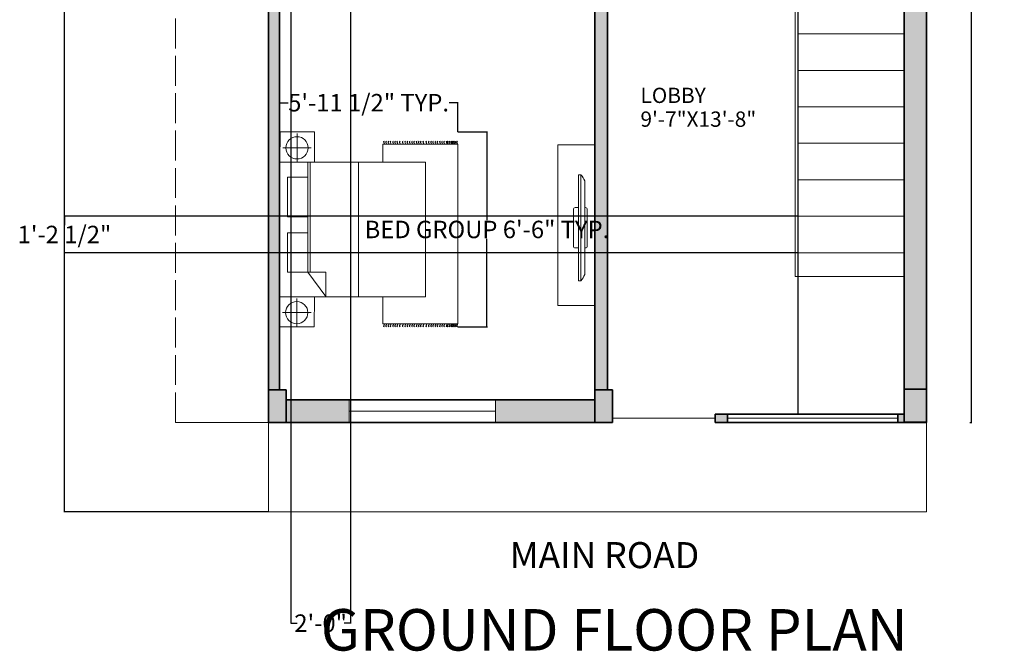
# Model space of a CAD drawing. Units: inches. Extents: x -17 to 892, y -721 to 172.
# Tile 1 of 11: x -17 to 378, y -715 to -462. Entities that reach past the tile are written whole.
import ezdxf

# ---------------------------------------------------------------- set-up
doc = ezdxf.new("R2010")
doc.units = ezdxf.units.IN
doc.header["$MEASUREMENT"] = 0
doc.linetypes.add('ACAD_ISO02W100', pattern=[15, 12, -3])
doc.layers.get('0').update_dxf_attribs({"color": 14})
for name, color, linetype, lineweight in [('A-ANNO-DIMS', 2, 'Continuous', 18), ('A-ANNO-TEXT', 7, 'Continuous', 18), ('A-ANNO-TITL', 7, 'Continuous', 35), ('A-AREA-IDEN', 7, 'Continuous', 18), ('A-COLS', 252, 'Continuous', 35), ('A-EQPM', 8, 'Continuous', 18), ('A-FLOR-CASE', 252, 'Continuous', 18), ('A-FLOR-STRS', 8, 'Continuous', 18), ('A-WALL-PATT', 14, 'Continuous', 13), ('C-PROP', 8, 'ACAD_ISO02W100', 18), ('C-ROAD', 8, 'Continuous', 18), ('doors', 4, 'Continuous', 18), ('furniture', 252, 'Continuous', 18), ('walls', 252, 'Continuous', 35), ('windows', 161, 'Continuous', 18)]:
    doc.layers.add(name, color=color, linetype=linetype, lineweight=lineweight)
doc.layers.add('A-COLS-PATT', color=254, linetype='Continuous', lineweight=13, true_color=0xd7ebd2)
doc.styles.get("Standard").update_dxf_attribs({"font": 'arial.ttf'})
doc.dimstyles.get("Standard").update_dxf_attribs({"dimtxt": 7, "dimasz": 0.18, "dimexe": 0.18, "dimexo": 0.0625, "dimgap": 0.09, "dimtad": 0, "dimtih": 1, "dimtoh": 1, "dimzin": 0, "dimdsep": 46, "dimlunit": 3, "dimtxsty": 'Standard', "dimcen": 0.09, "dimadec": 0, "dimazin": 0, "dimtfac": 1, "dimtofl": 0, "dimtmove": 0, "dimatfit": 3, "dimfxl": 1, "dimtolj": 1, "dimtzin": 0, "dimarcsym": 0})

# ---------------------------------------------------------------- blocks, each defined once
blk = doc.blocks.new('CARPET')
at = {"layer": 'furniture'}
for p, q in [((-51.53, -98.11), (-51.53, -55.12)), ((-51.53, -55.12), (-41.27, -55.12)), ((36, -55.12), (51.55, -55.12)), ((51.55, -55.12), (51.55, -98.11)), ((51.55, -98.11), (-51.53, -98.11))]:
    blk.add_line(p, q, dxfattribs=at)
for points, knots in [([(-53.37, -55.99), (-53.22, -55.8), (-52.9, -55.41), (-52.34, -55.8), (-51.89, -56.08), (-51.65, -55.91), (-51.53, -55.83)], [0, 0, 0, 0, 0.653278, 1.290138, 1.740457, 2.114451, 2.114451, 2.114451, 2.114451]), ([(53.37, -55.99), (53.22, -55.8), (52.9, -55.41), (52.34, -55.8), (51.89, -56.08), (51.65, -55.91), (51.53, -55.83)], [0, 0, 0, 0, 0.653278, 1.290138, 1.740457, 2.114451, 2.114451, 2.114451, 2.114451]), ([(-53.37, -57.26), (-53.22, -57.07), (-52.9, -56.67), (-52.34, -57.07), (-51.89, -57.35), (-51.65, -57.17), (-51.53, -57.1)], [0, 0, 0, 0, 0.653278, 1.290138, 1.740457, 2.114451, 2.114451, 2.114451, 2.114451]), ([(-53.37, -58.59), (-53.22, -58.4), (-52.9, -58.01), (-52.34, -58.4), (-51.89, -58.68), (-51.65, -58.5), (-51.53, -58.43)], [0, 0, 0, 0, 0.653278, 1.290138, 1.740457, 2.114451, 2.114451, 2.114451, 2.114451]), ([(-53.37, -59.78), (-53.22, -59.58), (-52.9, -59.19), (-52.34, -59.58), (-51.89, -59.86), (-51.65, -59.69), (-51.53, -59.61)], [0, 0, 0, 0, 0.653278, 1.290138, 1.740457, 2.114451, 2.114451, 2.114451, 2.114451]), ([(-53.37, -61.22), (-53.22, -61.02), (-52.9, -60.63), (-52.34, -61.02), (-51.89, -61.3), (-51.65, -61.13), (-51.53, -61.05)], [0, 0, 0, 0, 0.653278, 1.290138, 1.740457, 2.114451, 2.114451, 2.114451, 2.114451]), ([(-53.37, -62.44), (-53.22, -62.25), (-52.9, -61.86), (-52.34, -62.25), (-51.89, -62.53), (-51.65, -62.36), (-51.53, -62.28)], [0, 0, 0, 0, 0.653278, 1.290138, 1.740457, 2.114451, 2.114451, 2.114451, 2.114451]), ([(53.37, -57.26), (53.22, -57.07), (52.9, -56.67), (52.34, -57.07), (51.89, -57.35), (51.65, -57.17), (51.53, -57.1)], [0, 0, 0, 0, 0.653278, 1.290138, 1.740457, 2.114451, 2.114451, 2.114451, 2.114451]), ([(53.37, -58.59), (53.22, -58.4), (52.9, -58.01), (52.34, -58.4), (51.89, -58.68), (51.65, -58.5), (51.53, -58.43)], [0, 0, 0, 0, 0.653278, 1.290138, 1.740457, 2.114451, 2.114451, 2.114451, 2.114451]), ([(53.37, -59.78), (53.22, -59.58), (52.9, -59.19), (52.34, -59.58), (51.89, -59.86), (51.65, -59.69), (51.53, -59.61)], [0, 0, 0, 0, 0.653278, 1.290138, 1.740457, 2.114451, 2.114451, 2.114451, 2.114451]), ([(53.37, -61.22), (53.22, -61.02), (52.9, -60.63), (52.34, -61.02), (51.89, -61.3), (51.65, -61.13), (51.53, -61.05)], [0, 0, 0, 0, 0.653278, 1.290138, 1.740457, 2.114451, 2.114451, 2.114451, 2.114451]), ([(53.37, -62.44), (53.22, -62.25), (52.9, -61.86), (52.34, -62.25), (51.89, -62.53), (51.65, -62.36), (51.53, -62.28)], [0, 0, 0, 0, 0.653278, 1.290138, 1.740457, 2.114451, 2.114451, 2.114451, 2.114451]), ([(-53.37, -63.63), (-53.22, -63.43), (-52.9, -63.04), (-52.34, -63.43), (-51.89, -63.72), (-51.65, -63.54), (-51.53, -63.46)], [0, 0, 0, 0, 0.653278, 1.290138, 1.740457, 2.114451, 2.114451, 2.114451, 2.114451]), ([(-53.37, -65.07), (-53.22, -64.87), (-52.9, -64.48), (-52.34, -64.87), (-51.89, -65.15), (-51.65, -64.98), (-51.53, -64.9)], [0, 0, 0, 0, 0.653278, 1.290138, 1.740457, 2.114451, 2.114451, 2.114451, 2.114451]), ([(-53.37, -66.76), (-53.22, -66.56), (-52.9, -66.17), (-52.34, -66.56), (-51.89, -66.84), (-51.65, -66.67), (-51.53, -66.59)], [0, 0, 0, 0, 0.653278, 1.290138, 1.740457, 2.114451, 2.114451, 2.114451, 2.114451]), ([(-53.37, -68.2), (-53.22, -68), (-52.9, -67.61), (-52.34, -68), (-51.89, -68.28), (-51.65, -68.11), (-51.53, -68.03)], [0, 0, 0, 0, 0.653278, 1.290138, 1.740457, 2.114451, 2.114451, 2.114451, 2.114451]), ([(53.37, -63.63), (53.22, -63.43), (52.9, -63.04), (52.34, -63.43), (51.89, -63.72), (51.65, -63.54), (51.53, -63.46)], [0, 0, 0, 0, 0.653278, 1.290138, 1.740457, 2.114451, 2.114451, 2.114451, 2.114451]), ([(53.37, -65.07), (53.22, -64.87), (52.9, -64.48), (52.34, -64.87), (51.89, -65.15), (51.65, -64.98), (51.53, -64.9)], [0, 0, 0, 0, 0.653278, 1.290138, 1.740457, 2.114451, 2.114451, 2.114451, 2.114451]), ([(53.37, -66.76), (53.22, -66.56), (52.9, -66.17), (52.34, -66.56), (51.89, -66.84), (51.65, -66.67), (51.53, -66.59)], [0, 0, 0, 0, 0.653278, 1.290138, 1.740457, 2.114451, 2.114451, 2.114451, 2.114451]), ([(53.37, -68.2), (53.22, -68), (52.9, -67.61), (52.34, -68), (51.89, -68.28), (51.65, -68.11), (51.53, -68.03)], [0, 0, 0, 0, 0.653278, 1.290138, 1.740457, 2.114451, 2.114451, 2.114451, 2.114451]), ([(-53.37, -69.53), (-53.22, -69.33), (-52.9, -68.94), (-52.34, -69.33), (-51.89, -69.61), (-51.65, -69.44), (-51.53, -69.36)], [0, 0, 0, 0, 0.653278, 1.290138, 1.740457, 2.114451, 2.114451, 2.114451, 2.114451]), ([(-53.37, -70.79), (-53.22, -70.6), (-52.9, -70.21), (-52.34, -70.6), (-51.89, -70.88), (-51.65, -70.7), (-51.53, -70.63)], [0, 0, 0, 0, 0.653278, 1.290138, 1.740457, 2.114451, 2.114451, 2.114451, 2.114451]), ([(-53.37, -72.12), (-53.22, -71.93), (-52.9, -71.54), (-52.34, -71.93), (-51.89, -72.21), (-51.65, -72.04), (-51.53, -71.96)], [0, 0, 0, 0, 0.653278, 1.290138, 1.740457, 2.114451, 2.114451, 2.114451, 2.114451]), ([(-53.37, -73.31), (-53.22, -73.11), (-52.9, -72.72), (-52.34, -73.11), (-51.89, -73.4), (-51.65, -73.22), (-51.53, -73.14)], [0, 0, 0, 0, 0.653278, 1.290138, 1.740457, 2.114451, 2.114451, 2.114451, 2.114451]), ([(53.37, -69.53), (53.22, -69.33), (52.9, -68.94), (52.34, -69.33), (51.89, -69.61), (51.65, -69.44), (51.53, -69.36)], [0, 0, 0, 0, 0.653278, 1.290138, 1.740457, 2.114451, 2.114451, 2.114451, 2.114451]), ([(53.37, -70.79), (53.22, -70.6), (52.9, -70.21), (52.34, -70.6), (51.89, -70.88), (51.65, -70.7), (51.53, -70.63)], [0, 0, 0, 0, 0.653278, 1.290138, 1.740457, 2.114451, 2.114451, 2.114451, 2.114451]), ([(53.37, -72.12), (53.22, -71.93), (52.9, -71.54), (52.34, -71.93), (51.89, -72.21), (51.65, -72.04), (51.53, -71.96)], [0, 0, 0, 0, 0.653278, 1.290138, 1.740457, 2.114451, 2.114451, 2.114451, 2.114451]), ([(53.37, -73.31), (53.22, -73.11), (52.9, -72.72), (52.34, -73.11), (51.89, -73.4), (51.65, -73.22), (51.53, -73.14)], [0, 0, 0, 0, 0.653278, 1.290138, 1.740457, 2.114451, 2.114451, 2.114451, 2.114451]), ([(-53.37, -74.75), (-53.22, -74.55), (-52.9, -74.16), (-52.34, -74.55), (-51.89, -74.83), (-51.65, -74.66), (-51.53, -74.58)], [0, 0, 0, 0, 0.653278, 1.290138, 1.740457, 2.114451, 2.114451, 2.114451, 2.114451]), ([(-53.37, -75.98), (-53.22, -75.78), (-52.9, -75.39), (-52.34, -75.78), (-51.89, -76.06), (-51.65, -75.89), (-51.53, -75.81)], [0, 0, 0, 0, 0.653278, 1.290138, 1.740457, 2.114451, 2.114451, 2.114451, 2.114451]), ([(-53.37, -77.16), (-53.22, -76.96), (-52.9, -76.57), (-52.34, -76.96), (-51.89, -77.25), (-51.65, -77.07), (-51.53, -76.99)], [0, 0, 0, 0, 0.653278, 1.290138, 1.740457, 2.114451, 2.114451, 2.114451, 2.114451]), ([(-53.37, -78.6), (-53.22, -78.4), (-52.9, -78.01), (-52.34, -78.4), (-51.89, -78.68), (-51.65, -78.51), (-51.53, -78.43)], [0, 0, 0, 0, 0.653278, 1.290138, 1.740457, 2.114451, 2.114451, 2.114451, 2.114451]), ([(53.37, -74.75), (53.22, -74.55), (52.9, -74.16), (52.34, -74.55), (51.89, -74.83), (51.65, -74.66), (51.53, -74.58)], [0, 0, 0, 0, 0.653278, 1.290138, 1.740457, 2.114451, 2.114451, 2.114451, 2.114451]), ([(53.37, -75.98), (53.22, -75.78), (52.9, -75.39), (52.34, -75.78), (51.89, -76.06), (51.65, -75.89), (51.53, -75.81)], [0, 0, 0, 0, 0.653278, 1.290138, 1.740457, 2.114451, 2.114451, 2.114451, 2.114451]), ([(53.37, -77.16), (53.22, -76.96), (52.9, -76.57), (52.34, -76.96), (51.89, -77.25), (51.65, -77.07), (51.53, -76.99)], [0, 0, 0, 0, 0.653278, 1.290138, 1.740457, 2.114451, 2.114451, 2.114451, 2.114451]), ([(53.37, -78.6), (53.22, -78.4), (52.9, -78.01), (52.34, -78.4), (51.89, -78.68), (51.65, -78.51), (51.53, -78.43)], [0, 0, 0, 0, 0.653278, 1.290138, 1.740457, 2.114451, 2.114451, 2.114451, 2.114451]), ([(-53.37, -80.29), (-53.22, -80.09), (-52.9, -79.7), (-52.34, -80.09), (-51.89, -80.37), (-51.65, -80.2), (-51.53, -80.12)], [0, 0, 0, 0, 0.653278, 1.290138, 1.740457, 2.114451, 2.114451, 2.114451, 2.114451]), ([(-53.37, -81.73), (-53.22, -81.53), (-52.9, -81.14), (-52.34, -81.53), (-51.89, -81.81), (-51.65, -81.64), (-51.53, -81.56)], [0, 0, 0, 0, 0.653278, 1.290138, 1.740457, 2.114451, 2.114451, 2.114451, 2.114451]), ([(-53.37, -83.06), (-53.22, -82.86), (-52.9, -82.47), (-52.34, -82.86), (-51.89, -83.14), (-51.65, -82.97), (-51.53, -82.89)], [0, 0, 0, 0, 0.653278, 1.290138, 1.740457, 2.114451, 2.114451, 2.114451, 2.114451]), ([(-53.37, -84.18), (-53.22, -83.99), (-52.9, -83.6), (-52.34, -83.99), (-51.89, -84.27), (-51.65, -84.09), (-51.53, -84.02)], [0, 0, 0, 0, 0.653278, 1.290138, 1.740457, 2.114451, 2.114451, 2.114451, 2.114451]), ([(53.37, -80.29), (53.22, -80.09), (52.9, -79.7), (52.34, -80.09), (51.89, -80.37), (51.65, -80.2), (51.53, -80.12)], [0, 0, 0, 0, 0.653278, 1.290138, 1.740457, 2.114451, 2.114451, 2.114451, 2.114451]), ([(53.37, -81.73), (53.22, -81.53), (52.9, -81.14), (52.34, -81.53), (51.89, -81.81), (51.65, -81.64), (51.53, -81.56)], [0, 0, 0, 0, 0.653278, 1.290138, 1.740457, 2.114451, 2.114451, 2.114451, 2.114451]), ([(53.37, -83.06), (53.22, -82.86), (52.9, -82.47), (52.34, -82.86), (51.89, -83.14), (51.65, -82.97), (51.53, -82.89)], [0, 0, 0, 0, 0.653278, 1.290138, 1.740457, 2.114451, 2.114451, 2.114451, 2.114451]), ([(53.37, -84.18), (53.22, -83.99), (52.9, -83.6), (52.34, -83.99), (51.89, -84.27), (51.65, -84.09), (51.53, -84.02)], [0, 0, 0, 0, 0.653278, 1.290138, 1.740457, 2.114451, 2.114451, 2.114451, 2.114451]), ([(-53.37, -85.51), (-53.22, -85.32), (-52.9, -84.93), (-52.34, -85.32), (-51.89, -85.6), (-51.65, -85.42), (-51.53, -85.35)], [0, 0, 0, 0, 0.653278, 1.290138, 1.740457, 2.114451, 2.114451, 2.114451, 2.114451]), ([(-53.37, -86.7), (-53.22, -86.5), (-52.9, -86.11), (-52.34, -86.5), (-51.89, -86.78), (-51.65, -86.61), (-51.53, -86.53)], [0, 0, 0, 0, 0.653278, 1.290138, 1.740457, 2.114451, 2.114451, 2.114451, 2.114451]), ([(-53.37, -88.14), (-53.22, -87.94), (-52.9, -87.55), (-52.34, -87.94), (-51.89, -88.22), (-51.65, -88.05), (-51.53, -87.97)], [0, 0, 0, 0, 0.653278, 1.290138, 1.740457, 2.114451, 2.114451, 2.114451, 2.114451]), ([(-53.37, -89.36), (-53.22, -89.17), (-52.9, -88.78), (-52.34, -89.17), (-51.89, -89.45), (-51.65, -89.28), (-51.53, -89.2)], [0, 0, 0, 0, 0.653278, 1.290138, 1.740457, 2.114451, 2.114451, 2.114451, 2.114451]), ([(-53.37, -90.55), (-53.22, -90.35), (-52.9, -89.96), (-52.34, -90.35), (-51.89, -90.64), (-51.65, -90.46), (-51.53, -90.38)], [0, 0, 0, 0, 0.653278, 1.290138, 1.740457, 2.114451, 2.114451, 2.114451, 2.114451]), ([(53.37, -85.51), (53.22, -85.32), (52.9, -84.93), (52.34, -85.32), (51.89, -85.6), (51.65, -85.42), (51.53, -85.35)], [0, 0, 0, 0, 0.653278, 1.290138, 1.740457, 2.114451, 2.114451, 2.114451, 2.114451]), ([(53.37, -86.7), (53.22, -86.5), (52.9, -86.11), (52.34, -86.5), (51.89, -86.78), (51.65, -86.61), (51.53, -86.53)], [0, 0, 0, 0, 0.653278, 1.290138, 1.740457, 2.114451, 2.114451, 2.114451, 2.114451]), ([(53.37, -88.14), (53.22, -87.94), (52.9, -87.55), (52.34, -87.94), (51.89, -88.22), (51.65, -88.05), (51.53, -87.97)], [0, 0, 0, 0, 0.653278, 1.290138, 1.740457, 2.114451, 2.114451, 2.114451, 2.114451]), ([(53.37, -89.36), (53.22, -89.17), (52.9, -88.78), (52.34, -89.17), (51.89, -89.45), (51.65, -89.28), (51.53, -89.2)], [0, 0, 0, 0, 0.653278, 1.290138, 1.740457, 2.114451, 2.114451, 2.114451, 2.114451]), ([(53.37, -90.55), (53.22, -90.35), (52.9, -89.96), (52.34, -90.35), (51.9, -90.63), (51.66, -90.47), (51.55, -90.4)], [0, 0, 0, 0, 0.653278, 1.290138, 1.740457, 2.0926, 2.0926, 2.0926, 2.0926]), ([(-53.37, -91.99), (-53.22, -91.79), (-52.9, -91.4), (-52.34, -91.79), (-51.89, -92.07), (-51.65, -91.9), (-51.53, -91.82)], [0, 0, 0, 0, 0.653278, 1.290138, 1.740457, 2.114451, 2.114451, 2.114451, 2.114451]), ([(-53.37, -92.69), (-53.22, -92.48), (-52.9, -92.08), (-52.35, -92.49), (-51.89, -92.77), (-51.65, -92.6), (-51.53, -92.52)], [0, 0, 0, 0, 0.663904, 1.307406, 1.757725, 2.131719, 2.131719, 2.131719, 2.131719]), ([(-53.37, -93.61), (-53.22, -93.42), (-52.9, -93.03), (-52.34, -93.42), (-51.89, -93.7), (-51.65, -93.52), (-51.53, -93.45)], [0, 0, 0, 0, 0.653278, 1.290138, 1.740457, 2.114451, 2.114451, 2.114451, 2.114451]), ([(-53.37, -94.55), (-53.22, -94.35), (-52.9, -93.96), (-52.34, -94.35), (-51.89, -94.63), (-51.65, -94.46), (-51.53, -94.38)], [0, 0, 0, 0, 0.653278, 1.290138, 1.740457, 2.114451, 2.114451, 2.114451, 2.114451]), ([(-53.37, -95.05), (-53.22, -94.85), (-52.9, -94.46), (-52.34, -94.85), (-51.89, -95.14), (-51.65, -94.96), (-51.53, -94.88)], [0, 0, 0, 0, 0.653278, 1.290138, 1.740457, 2.114451, 2.114451, 2.114451, 2.114451]), ([(-53.37, -95.73), (-53.22, -95.54), (-52.9, -95.15), (-52.34, -95.54), (-51.89, -95.82), (-51.65, -95.65), (-51.53, -95.57)], [0, 0, 0, 0, 0.653278, 1.290138, 1.740457, 2.114451, 2.114451, 2.114451, 2.114451]), ([(-53.37, -96.38), (-53.22, -96.18), (-52.9, -95.79), (-52.34, -96.18), (-51.89, -96.47), (-51.65, -96.29), (-51.53, -96.21)], [0, 0, 0, 0, 0.653278, 1.290138, 1.740457, 2.114451, 2.114451, 2.114451, 2.114451]), ([(53.37, -95.78), (53.22, -95.58), (52.9, -95.19), (52.34, -95.58), (51.89, -95.86), (51.65, -95.69), (51.53, -95.61)], [0, 0, 0, 0, 0.653278, 1.290138, 1.740457, 2.114451, 2.114451, 2.114451, 2.114451]), ([(53.37, -96.43), (53.22, -96.23), (52.9, -95.84), (52.34, -96.23), (51.89, -96.51), (51.65, -96.34), (51.53, -96.26)], [0, 0, 0, 0, 0.653278, 1.290138, 1.740457, 2.114451, 2.114451, 2.114451, 2.114451]), ([(53.37, -91.99), (53.22, -91.79), (52.9, -91.4), (52.34, -91.79), (51.9, -92.07), (51.66, -91.91), (51.55, -91.83)], [0, 0, 0, 0, 0.653278, 1.290138, 1.740457, 2.0926, 2.0926, 2.0926, 2.0926]), ([(53.37, -92.69), (53.22, -92.49), (52.9, -92.09), (52.34, -92.49), (51.9, -92.77), (51.66, -92.61), (51.55, -92.53)], [0, 0, 0, 0, 0.656792, 1.295826, 1.746145, 2.098292, 2.098292, 2.098292, 2.098292]), ([(53.37, -93.66), (53.22, -93.46), (52.9, -93.07), (52.34, -93.46), (51.9, -93.74), (51.66, -93.58), (51.55, -93.5)], [0, 0, 0, 0, 0.653278, 1.290138, 1.740457, 2.0926, 2.0926, 2.0926, 2.0926]), ([(53.37, -94.59), (53.22, -94.4), (52.9, -94.01), (52.34, -94.4), (51.9, -94.68), (51.66, -94.51), (51.55, -94.44)], [0, 0, 0, 0, 0.653278, 1.290138, 1.740457, 2.0926, 2.0926, 2.0926, 2.0926]), ([(53.37, -95.1), (53.22, -94.9), (52.9, -94.51), (52.34, -94.9), (51.9, -95.18), (51.66, -95.02), (51.55, -94.94)], [0, 0, 0, 0, 0.653278, 1.290138, 1.740457, 2.0926, 2.0926, 2.0926, 2.0926]), ([(-53.37, -97.17), (-53.22, -96.98), (-52.9, -96.59), (-52.34, -96.98), (-51.89, -97.26), (-51.65, -97.08), (-51.53, -97.01)], [0, 0, 0, 0, 0.653278, 1.290138, 1.740457, 2.114451, 2.114451, 2.114451, 2.114451]), ([(-53.37, -97.99), (-53.22, -97.79), (-52.9, -97.4), (-52.34, -97.79), (-51.89, -98.08), (-51.65, -97.9), (-51.53, -97.82)], [0, 0, 0, 0, 0.653278, 1.290138, 1.740457, 2.114451, 2.114451, 2.114451, 2.114451]), ([(53.37, -97.22), (53.22, -97.02), (52.9, -96.63), (52.34, -97.02), (51.89, -97.3), (51.65, -97.13), (51.53, -97.05)], [0, 0, 0, 0, 0.653278, 1.290138, 1.740457, 2.114451, 2.114451, 2.114451, 2.114451]), ([(53.37, -97.99), (53.22, -97.79), (52.9, -97.4), (52.34, -97.79), (51.89, -98.08), (51.65, -97.9), (51.53, -97.82)], [0, 0, 0, 0, 0.653278, 1.290138, 1.740457, 2.114451, 2.114451, 2.114451, 2.114451])]:
    blk.add_open_spline(points, degree=3, knots=knots, dxfattribs=at)
blk = doc.blocks.new('A$C58D270C6')
at = {"layer": 'furniture'}
for p, q in [((9.09, 124.13), (9.09, 108.87)), ((1.46, 116.5), (16.73, 116.5)), ((14.97, 94.84), (24.62, 107.92)), ((24.62, 94.93), (24.62, 107.92)), ((42.08, 108), (42.08, 36)), ((14.97, 94.93), (24.62, 94.93)), ((14.97, 94.84), (14.97, 36)), ((16.22, 94.93), (16.22, 36)), ((9.25, 36), (9.25, 20.74)), ((1.62, 28.37), (16.88, 28.37))]:
    blk.add_line(p, q, dxfattribs=at)
for points in [[(18.5, 108), (18.34, 124.13), (-0.16, 124.13), (0, 108)], [(0, 108), (77.91, 108), (77.91, 36), (0, 36)], [(4.09, 94.93), (14.97, 94.93), (14.97, 73.83), (4.09, 73.83)], [(4.09, 65.23), (14.97, 65.23), (14.97, 44.13), (4.09, 44.13)], [(18.65, 19.87), (18.5, 36), (0, 36), (0.16, 19.87)]]:
    blk.add_lwpolyline(points, close=True, dxfattribs=at)
for centre in [(9.09, 116.5), (9.25, 28.37)]:
    blk.add_circle(centre, 5.95, dxfattribs=at)
at = {"layer": 'furniture', "xscale": 0.9312884925094044, "yscale": 0.9312884925094044, "zscale": 0.9312884925094044, "rotation": 90}
blk.add_blockref('CARPET', (3.79, 74.47), dxfattribs=at)
blk = doc.blocks.new('PLASMA-LARGE')
at = {"layer": 'furniture'}
for p, q in [((-7.26, 0), (7.26, 0)), ((-21, -2.5), (21, -2.5)), ((-21, -2.5), (-21, -3.5)), ((-21, -3.5), (21, -3.5)), ((-18.61, -1), (18.61, -1)), ((-8, -1), (-8, -0.74)), ((-8, -3.5), (-8, -4.76)), ((8, -1), (8, -0.74)), ((8, -3.5), (8, -4.76)), ((21, -2.5), (21, -3.5)), ((-7.26, -5.5), (7.26, -5.5))]:
    blk.add_line(p, q, dxfattribs=at)
for centre, radius, start, end in [((-7.26, -0.74), 0.744, 90, 180), ((7.26, -0.74), 0.744, 0, 90), ((-13.97, -11.05), 11.07, 114.7602, 129.4175), ((13.97, -11.05), 11.07, 50.5825, 65.2398), ((-7.26, -4.76), 0.744, 180, 270), ((7.26, -4.76), 0.744, 270, 0)]:
    blk.add_arc(centre, radius, start, end, dxfattribs=at)
blk = doc.blocks.new('*D16')
at = {"layer": 'A-ANNO-DIMS', "color": 0, "lineweight": -2, "transparency": 16777216}
for p, q in [((364.49, 89.9), (365.24, 89.9)), ((365.06, 89.72), (365.06, -263.08)), ((365.06, -623.21), (365.06, -270.41)), ((364.49, -623.39), (365.24, -623.39))]:
    blk.add_line(p, q, dxfattribs=at)
at = {"layer": 'A-ANNO-DIMS', "color": 0, "lineweight": 100, "transparency": 16777216}
for points in [[(365.03, 89.72), (365.09, 89.72), (365.06, 89.9)], [(365.03, -623.21), (365.09, -623.21), (365.06, -623.39)]]:
    blk.add_solid(points, dxfattribs=at)
at = {"layer": 'Defpoints', "color": 0, "lineweight": 100, "transparency": 16777216}
for p in [(364.43, 89.9), (364.43, -623.39), (365.06, -623.39)]:
    blk.add_point(p, dxfattribs=at)
at = {"layer": 'A-ANNO-DIMS', "color": 0, "transparency": 16777216, "insert": (365.06, -266.74), "char_height": 7, "attachment_point": 5}
blk.add_mtext('\\A1;57\'-1"', dxfattribs=at)
blk = doc.blocks.new('MEDIA-CONSOLE')
for p, q in [((14.9, 64.44), (0, 64.44)), ((14.9, 0), (14.9, 64.44)), ((0, 0), (14.9, 0))]:
    blk.add_line(p, q)
blk = doc.blocks.new('*D30')
at = {"layer": 'A-ANNO-DIMS', "color": 0, "lineweight": -2, "transparency": 16777216}
for p, q in [((159.08, -506.9), (170.94, -506.9)), ((170.76, -507.08), (170.76, -542.31)), ((170.76, -584.95), (170.76, -549.73)), ((159.08, -585.13), (170.94, -585.13))]:
    blk.add_line(p, q, dxfattribs=at)
at = {"layer": 'A-ANNO-DIMS', "color": 0, "lineweight": 100, "transparency": 16777216}
for points in [[(170.73, -507.08), (170.79, -507.08), (170.76, -506.9)], [(170.73, -584.95), (170.79, -584.95), (170.76, -585.13)]]:
    blk.add_solid(points, dxfattribs=at)
at = {"layer": 'Defpoints', "color": 0, "lineweight": 100, "transparency": 16777216}
for p in [(159.02, -506.9), (159.02, -585.13), (170.76, -585.13)]:
    blk.add_point(p, dxfattribs=at)
at = {"layer": 'A-ANNO-DIMS', "color": 0, "transparency": 16777216, "insert": (170.76, -546.02), "char_height": 7, "attachment_point": 5}
blk.add_mtext('\\A1;BED GROUP 6\'-6" TYP.', dxfattribs=at)
blk = doc.blocks.new('*D31')
at = {"layer": 'A-ANNO-DIMS', "color": 0, "lineweight": -2, "transparency": 16777216}
for p, q in [((87.54, -506.84), (87.54, -494.99)), ((87.72, -495.17), (90.98, -495.17)), ((158.84, -495.17), (155.58, -495.17)), ((159.02, -506.84), (159.02, -494.99))]:
    blk.add_line(p, q, dxfattribs=at)
at = {"layer": 'A-ANNO-DIMS', "color": 0, "lineweight": 100, "transparency": 16777216}
for points in [[(87.72, -495.14), (87.72, -495.2), (87.54, -495.17)], [(158.84, -495.14), (158.84, -495.2), (159.02, -495.17)]]:
    blk.add_solid(points, dxfattribs=at)
at = {"layer": 'Defpoints', "color": 0, "lineweight": 100, "transparency": 16777216}
for p in [(159.02, -495.17), (87.54, -506.9), (159.02, -506.9)]:
    blk.add_point(p, dxfattribs=at)
at = {"layer": 'A-ANNO-DIMS', "color": 0, "transparency": 16777216, "insert": (123.28, -495.17), "char_height": 7, "attachment_point": 5}
blk.add_mtext('\\A1;5\'-11 1/2" TYP.', dxfattribs=at)
blk = doc.blocks.new('*D57')
at = {"layer": 'A-ANNO-DIMS', "color": 0, "lineweight": -2, "transparency": 16777216}
for p, q in [((83.02, 89.9), (1.11, 89.9)), ((1.29, 89.72), (1.29, -281.05)), ((1.29, -659.16), (1.29, -288.38)), ((83.02, -659.34), (1.11, -659.34))]:
    blk.add_line(p, q, dxfattribs=at)
at = {"layer": 'A-ANNO-DIMS', "color": 0, "lineweight": 100, "transparency": 16777216}
for points in [[(1.26, 89.72), (1.32, 89.72), (1.29, 89.9)], [(1.26, -659.16), (1.32, -659.16), (1.29, -659.34)]]:
    blk.add_solid(points, dxfattribs=at)
at = {"layer": 'Defpoints', "color": 0, "lineweight": 100, "transparency": 16777216}
for p in [(1.29, 89.9), (83.08, 89.9), (83.08, -659.34)]:
    blk.add_point(p, dxfattribs=at)
at = {"layer": 'A-ANNO-DIMS', "color": 0, "transparency": 16777216, "insert": (1.29, -284.72), "char_height": 7, "attachment_point": 5}
blk.add_mtext('\\A1;62\'-5"', dxfattribs=at)
blk = doc.blocks.new('*D60')
at = {"layer": 'A-ANNO-DIMS', "color": 0, "lineweight": -2, "transparency": 16777216}
for p, q in [((116.03, -326.38), (116.03, -704.12)), ((92.08, -351.45), (92.08, -704.12)), ((92.26, -703.94), (94.6, -703.94)), ((115.85, -703.94), (113.51, -703.94))]:
    blk.add_line(p, q, dxfattribs=at)
at = {"layer": 'A-ANNO-DIMS', "color": 0, "lineweight": 100, "transparency": 16777216}
for points in [[(92.26, -703.91), (92.26, -703.97), (92.08, -703.94)], [(115.85, -703.91), (115.85, -703.97), (116.03, -703.94)]]:
    blk.add_solid(points, dxfattribs=at)
at = {"layer": 'Defpoints', "color": 0, "lineweight": 100, "transparency": 16777216}
for p in [(116.03, -326.32), (92.08, -351.39), (116.03, -703.94)]:
    blk.add_point(p, dxfattribs=at)
at = {"layer": 'A-ANNO-DIMS', "color": 0, "transparency": 16777216, "insert": (104.05, -703.94), "char_height": 7, "attachment_point": 5}
blk.add_mtext('\\A1;2\'-0"', dxfattribs=at)
blk = doc.blocks.new('*D63')
at = {"layer": 'A-ANNO-DIMS', "color": 0, "lineweight": -2, "transparency": 16777216}
for p, q in [((295.55, -619.99), (295.55, 161.84)), ((295.73, 161.66), (299.27, 161.66)), ((337.9, 161.66), (334.36, 161.66)), ((338.08, -619.99), (338.08, 161.84))]:
    blk.add_line(p, q, dxfattribs=at)
at = {"layer": 'A-ANNO-DIMS', "color": 0, "lineweight": 100, "transparency": 16777216}
for points in [[(295.73, 161.69), (295.73, 161.63), (295.55, 161.66)], [(337.9, 161.69), (337.9, 161.63), (338.08, 161.66)]]:
    blk.add_solid(points, dxfattribs=at)
at = {"layer": 'Defpoints', "color": 0, "lineweight": 100, "transparency": 16777216}
for p in [(338.08, 161.66), (295.55, -620.06), (338.08, -620.06)]:
    blk.add_point(p, dxfattribs=at)
at = {"layer": 'A-ANNO-DIMS', "color": 0, "transparency": 16777216, "insert": (316.82, 161.66), "char_height": 7, "attachment_point": 5}
blk.add_mtext('\\A1;3\'-6 1/2"', dxfattribs=at)
blk = doc.blocks.new('*D64')
at = {"layer": 'A-ANNO-DIMS', "color": 0, "lineweight": -2, "transparency": 16777216}
for p, q in [((295.49, -540.72), (1.11, -540.72)), ((1.29, -540.9), (1.29, -544.33)), ((1.29, -555.17), (1.29, -551.75)), ((295.49, -555.35), (1.11, -555.35))]:
    blk.add_line(p, q, dxfattribs=at)
at = {"layer": 'A-ANNO-DIMS', "color": 0, "lineweight": 100, "transparency": 16777216}
for points in [[(1.26, -540.9), (1.32, -540.9), (1.29, -540.72)], [(1.26, -555.17), (1.32, -555.17), (1.29, -555.35)]]:
    blk.add_solid(points, dxfattribs=at)
at = {"layer": 'Defpoints', "color": 0, "lineweight": 100, "transparency": 16777216}
for p in [(1.29, -540.72), (295.55, -540.72), (295.55, -555.35)]:
    blk.add_point(p, dxfattribs=at)
at = {"layer": 'A-ANNO-DIMS', "color": 0, "transparency": 16777216, "insert": (1.29, -548.04), "char_height": 7, "attachment_point": 5}
blk.add_mtext('\\A1;1\'-2 1/2"', dxfattribs=at)

msp = doc.modelspace()

# ---------------------------------------------------------------- hatches: boundary and pattern name
at = {"layer": 'A-COLS-PATT'}
h = msp.add_hatch(color=256, dxfattribs=at)
h.dxf.hatch_style = 1
h.paths.add_polyline_path([(92.084, 61.611), (83.084, 61.611), (83.084, 43.692), (92.084, 43.692)])
h.paths.add_polyline_path([(347.084, 61.611), (338.084, 61.611), (338.084, 43.692), (347.084, 43.692)])
h.paths.add_polyline_path([(222.053, 61.611), (209.95, 61.611), (209.95, 52.611), (222.053, 52.611)])
h.paths.add_polyline_path([(284.798, 61.611), (274.584, 61.611), (274.584, 52.611), (284.798, 52.611)])
h.paths.add_polyline_path([(223.084, -106.389), (214.084, -106.389), (214.084, -119.959), (223.084, -119.959)])
h.paths.add_polyline_path([(347.084, -148.653), (338.084, -148.653), (338.084, -172.24), (347.084, -172.24)])
h.paths.add_polyline_path([(92.084, -102.402), (83.084, -102.402), (83.084, -119.959), (92.084, -119.959)])
h.paths.add_polyline_path([(92.084, -205.889), (83.084, -205.889), (83.084, -216.319), (92.084, -216.319)])
h.paths.add_polyline_path([(347.084, -349.073), (338.084, -349.073), (338.084, -372.66), (347.084, -372.66)])
h.paths.add_polyline_path([(347.084, -610.134), (338.084, -610.134), (338.084, -614.389), (338.084, -623.342), (347.084, -623.342)])
h.paths.add_polyline_path([(221.166, -610.357), (214.084, -610.357), (214.084, -623.389), (219.084, -623.389), (221.166, -623.389), (221.166, -621.723)])
h.paths.add_polyline_path([(90.166, -610.357), (83.084, -610.357), (83.084, -623.389), (90.166, -623.389)])
h.paths.add_polyline_path([(223.084, -401.64), (214.084, -401.64), (214.084, -410.389), (223.084, -410.389)])
h.paths.add_polyline_path([(223.084, -356.889), (214.084, -356.889), (214.084, -369.273), (223.084, -369.273)])
h.paths.add_polyline_path([(92.084, -398.492), (83.084, -398.492), (83.084, -410.389), (92.084, -410.389)])
h.paths.add_polyline_path([(92.084, -348.918), (83.084, -348.918), (83.084, -360.706), (92.084, -360.706)])
at = {"layer": 'A-WALL-PATT'}
h = msp.add_hatch(color=256, dxfattribs=at)
h.dxf.hatch_style = 1
h.paths.add_polyline_path([(111.26, 61.611), (92.084, 61.611), (92.084, 52.611), (111.26, 52.611)])
h.paths.add_polyline_path([(209.95, 61.611), (179.154, 61.611), (179.154, 52.611), (209.95, 52.611)])
h.paths.add_polyline_path([(338.084, 61.611), (284.798, 61.611), (284.798, 52.611), (338.084, 52.611)])
h.paths.add_polyline_path([(279.084, 23.861), (274.584, 23.861), (274.584, -0.389), (279.084, -0.389)])
h.paths.add_polyline_path([(279.084, 52.611), (274.584, 52.611), (274.584, 46.881), (276.834, 46.881), (279.084, 46.881)])
h.paths.add_polyline_path([(279.084, -0.389), (274.584, -0.389), (274.584, -4.889), (279.084, -4.889)])
h.paths.add_polyline_path([(304.22, -0.389), (279.084, -0.389), (279.084, -4.889), (304.22, -4.889)])
h.paths.add_polyline_path([(347.084, 43.692), (338.084, 43.692), (338.084, -148.653), (347.084, -148.653)])
h.paths.add_polyline_path([(338.084, -154.889), (264.103, -154.889), (264.103, -163.889), (338.084, -163.889)])
h.paths.add_polyline_path([(223.084, -119.959), (214.084, -119.959), (214.084, -163.889), (223.084, -163.889)])
h.paths.add_polyline_path([(218.584, 52.611), (214.084, 52.611), (214.084, -106.389), (218.584, -106.389)])
h.paths.add_polyline_path([(92.084, -8.943), (83.084, -8.943), (83.084, -49.69), (87.584, -49.69), (92.084, -49.69)])
h.paths.add_polyline_path([(92.084, 43.692), (83.084, 43.692), (83.084, 33.018), (87.584, 33.018), (92.084, 33.018)])
h.paths.add_polyline_path([(92.084, -91.651), (83.084, -91.651), (83.084, -102.402), (92.084, -102.402)])
h.paths.add_polyline_path([(92.084, -119.959), (83.084, -119.959), (83.084, -151.855), (87.584, -151.855), (92.084, -151.855)])
h.paths.add_polyline_path([(173.584, -108.639), (173.584, -106.389), (173.084, -106.389), (92.084, -106.389), (92.084, -110.889), (169.084, -110.889), (169.084, -176.029), (173.584, -176.029)])
h.paths.add_polyline_path([(92.084, -185.221), (83.084, -185.221), (83.084, -205.889), (92.084, -205.889)])
h.paths.add_polyline_path([(92.084, -216.319), (83.084, -216.319), (83.084, -259.015), (87.584, -259.015), (92.084, -259.015)])
h.paths.add_polyline_path([(173.584, -205.889), (92.084, -205.889), (92.084, -210.389), (169.084, -210.389), (169.084, -236.193), (173.584, -236.193)])
h.paths.add_polyline_path([(92.084, -300.976), (83.084, -300.976), (83.084, -348.918), (92.084, -348.918)])
h.paths.add_polyline_path([(87.584, -410.389), (83.084, -410.389), (83.084, -610.357), (87.584, -610.357)])
h.paths.add_polyline_path([(115.523, -614.389), (90.166, -614.389), (90.166, -623.389), (115.523, -623.389)])
h.paths.add_polyline_path([(214.084, -614.389), (174.149, -614.389), (174.149, -623.389), (214.084, -623.389)])
h.paths.add_polyline_path([(219.084, -410.389), (214.084, -410.389), (214.084, -610.357), (219.084, -610.357)])
h.paths.add_polyline_path([(347.084, -372.66), (338.084, -372.66), (338.084, -610.134), (347.084, -610.134)])
h.paths.add_polyline_path([(347.084, -172.24), (338.084, -172.24), (338.084, -349.073), (347.084, -349.073)])
h.paths.add_polyline_path([(338.084, -356.889), (317.618, -356.889), (317.618, -365.889), (338.084, -365.889)])
h.paths.add_polyline_path([(267.632, -356.889), (263.828, -356.889), (263.828, -365.889), (267.632, -365.889)])
h.paths.add_polyline_path([(223.084, -369.273), (214.084, -369.273), (214.084, -401.64), (223.084, -401.64)])
h = msp.add_hatch(color=256, dxfattribs=at)
h.dxf.hatch_style = 1
h.paths.add_polyline_path([(267.203, -620.057), (262.274, -620.057), (262.274, -623.389), (267.203, -623.389)])
h.paths.add_polyline_path([(338.084, -620.057), (335.531, -620.057), (335.531, -623.389), (338.084, -623.389)])
h.paths.add_polyline_path([(173.584, -405.889), (153.584, -405.889), (153.584, -396.835), (149.084, -396.835), (149.084, -405.889), (92.084, -405.889), (92.084, -410.389), (173.584, -410.389)])
h.paths.add_polyline_path([(153.584, -355.889), (173.584, -355.889), (173.584, -320.35), (169.084, -320.35), (169.084, -351.389), (92.084, -351.389), (92.084, -355.889), (149.084, -355.889), (149.084, -364.083), (153.584, -364.083)])

# ---------------------------------------------------------------- linework, layer by layer
at = {"layer": 'A-COLS'}
for p, q in [((83.084, -610.357), (90.166, -610.357)), ((90.166, -610.357), (90.166, -623.389)), ((214.084, -610.357), (221.166, -610.357)), ((221.166, -610.357), (221.166, -621.723)), ((338.084, -610.134), (347.084, -610.134)), ((338.084, -623.342), (338.084, -614.389)), ((219.084, -623.389), (221.166, -623.389)), ((221.166, -623.389), (221.166, -621.723)), ((338.084, -623.342), (347.084, -623.342))]:
    msp.add_line(p, q, dxfattribs=at)
at = {"layer": 'A-FLOR-STRS'}
for p, q in [((295.55, -394.434), (295.55, -620.057)), ((294.357, -395.993), (294.357, -564.936)), ((295.55, -467.579), (338.084, -467.579)), ((295.55, -482.207), (338.084, -482.207)), ((295.55, -496.836), (338.084, -496.836)), ((295.55, -511.465), (338.084, -511.465)), ((295.55, -526.094), (338.084, -526.094)), ((295.55, -540.723), (338.084, -540.723)), ((295.55, -555.352), (338.084, -555.352)), ((294.357, -564.936), (338.084, -564.936))]:
    msp.add_line(p, q, dxfattribs=at)
at = {"layer": 'C-PROP'}
msp.add_line((45.892, -623.389), (45.892, 61.611), dxfattribs=at)
at = {"layer": 'C-ROAD'}
for p, q in [((83.084, -623.389), (45.892, -623.389)), ((83.084, -623.389), (83.084, -659.336)), ((347.084, -659.336), (347.084, -623.389)), ((83.084, -659.336), (347.084, -659.336))]:
    msp.add_line(p, q, dxfattribs=at)
at = {"layer": 'doors'}
msp.add_line((262.274, -621.723), (221.166, -621.723), dxfattribs=at)
at = {"layer": 'walls'}
for p, q in [((83.084, -623.389), (83.084, 61.611)), ((338.084, 61.611), (338.084, -614.389)), ((347.084, 61.611), (347.084, -623.389)), ((214.084, -623.389), (214.084, -356.889)), ((87.584, -610.357), (87.584, -410.389)), ((219.084, -610.357), (219.084, -410.389)), ((214.084, -614.389), (90.166, -614.389)), ((219.084, -623.389), (83.084, -623.389)), ((262.274, -623.389), (262.274, -620.057)), ((262.274, -620.057), (338.084, -620.057)), ((347.084, -623.389), (262.274, -623.389)), ((267.203, -623.389), (267.203, -620.057)), ((335.531, -620.057), (335.531, -623.389))]:
    msp.add_line(p, q, dxfattribs=at)
at = {"layer": 'windows'}
for p, q in [((115.523, -614.389), (115.523, -623.389)), ((174.149, -614.389), (115.523, -614.389)), ((115.523, -614.389), (115.523, -618.889)), ((174.149, -623.389), (174.149, -614.389)), ((115.523, -618.889), (174.149, -618.889)), ((115.523, -623.389), (174.149, -623.389)), ((267.203, -621.723), (335.531, -621.723))]:
    msp.add_line(p, q, dxfattribs=at)

# ---------------------------------------------------------------- block references
at = {"layer": 'A-EQPM', "xscale": 1.011294184530666, "yscale": 1.011294184530666, "zscale": 1.011294184530666, "rotation": 270}
msp.add_blockref('PLASMA-LARGE', (210.973, -545.326), dxfattribs=at)
at = {"layer": 'A-FLOR-CASE', "rotation": 180}
msp.add_blockref('MEDIA-CONSOLE', (214.084, -512.065), dxfattribs=at)
at = {"layer": 'furniture', "xscale": -0.7500000390647866, "yscale": 0.7500000390647866, "zscale": 0.7500000390647866, "rotation": 180}
msp.add_blockref('A$C58D270C6', (87.653, -492), dxfattribs=at)

# ---------------------------------------------------------------- texts
at = {"layer": 'A-ANNO-TEXT'}
msp.add_text('MAIN ROAD', height=10.4498, dxfattribs=at).set_placement((179.874, -681.884))
at = {"layer": 'A-ANNO-TITL'}
msp.add_text('GROUND FLOOR PLAN', height=16.63981, dxfattribs=at).set_placement((104.16, -714.943))
at = {"layer": 'A-AREA-IDEN'}
for s, p in [('LOBBY', (232.322, -495.301)), ('9\'-7"X13\'-8"', (232.322, -504.836))]:
    msp.add_text(s, height=6.1361, dxfattribs=at).set_placement(p)

# ---------------------------------------------------------------- dimensions: what is measured, and where the dimension line sits
at = {"layer": 'A-ANNO-DIMS'}
for base, p1, p2, picture, middle in [((338.084, 161.663), (295.55, -620.057), (338.084, -620.057), '*D63', (316.817, 161.663)), ((116.026, -703.936), (92.084, -351.389), (116.026, -326.317), '*D60', (104.055, -703.936))]:
    dim = msp.add_linear_dim(base=base, p1=p1, p2=p2, dimstyle='Standard', override={"dimdec": 1, "dimlfac": 1, "dimrnd": 0, "dimzin": 1, "dimdsep": 46, "dimlunit": 4, "dimfrac": 2}, dxfattribs=at)
    dim.commit()
    dim.dimension.update_dxf_attribs({"geometry": picture, "text_midpoint": middle})
for base, p1, p2, picture, middle in [((1.292, 89.902), (83.084, -659.336), (83.084, 89.902), '*D57', (1.292, -284.717)), ((1.292, -540.723), (295.55, -555.352), (295.55, -540.723), '*D64', (1.292, -548.037))]:
    dim = msp.add_linear_dim(base=base, p1=p1, p2=p2, angle=90, dimstyle='Standard', override={"dimdec": 1, "dimlfac": 1, "dimrnd": 0, "dimzin": 1, "dimdsep": 46, "dimlunit": 4, "dimfrac": 2}, dxfattribs=at)
    dim.commit()
    dim.dimension.update_dxf_attribs({"geometry": picture, "text_midpoint": middle})
for base, p1, p2, angle, text, override, picture, middle in [((365.057, -623.389), (364.432, 89.902), (364.432, -623.389), 90, '57\'-1"', {"dimclrd": 0, "dimclre": 0, "dimclrt": 0}, '*D16', (365.057, -266.744)), ((170.757, -585.135), (159.022, -506.901), (159.022, -585.135), 270, 'BED GROUP <> TYP.', {"dimdec": 1, "dimlfac": 1, "dimrnd": 0, "dimzin": 1, "dimdsep": 46, "dimlunit": 4, "dimfrac": 2}, '*D30', (170.757, -546.018))]:
    dim = msp.add_linear_dim(base=base, p1=p1, p2=p2, angle=angle, text=text, dimstyle='Standard', override=override, dxfattribs=at)
    dim.commit()
    dim.dimension.update_dxf_attribs({"geometry": picture, "text_midpoint": middle})
dim = msp.add_linear_dim(base=(159.022, -495.166), p1=(87.537, -506.901), p2=(159.022, -506.901), text='<> TYP.', dimstyle='Standard', override={"dimdec": 1, "dimlfac": 1, "dimrnd": 0, "dimzin": 1, "dimdsep": 46, "dimlunit": 4, "dimfrac": 2}, dxfattribs=at)
dim.commit()
dim.dimension.update_dxf_attribs({"geometry": '*D31', "text_midpoint": (123.28, -495.166)})

doc.saveas('drawing.dxf')
